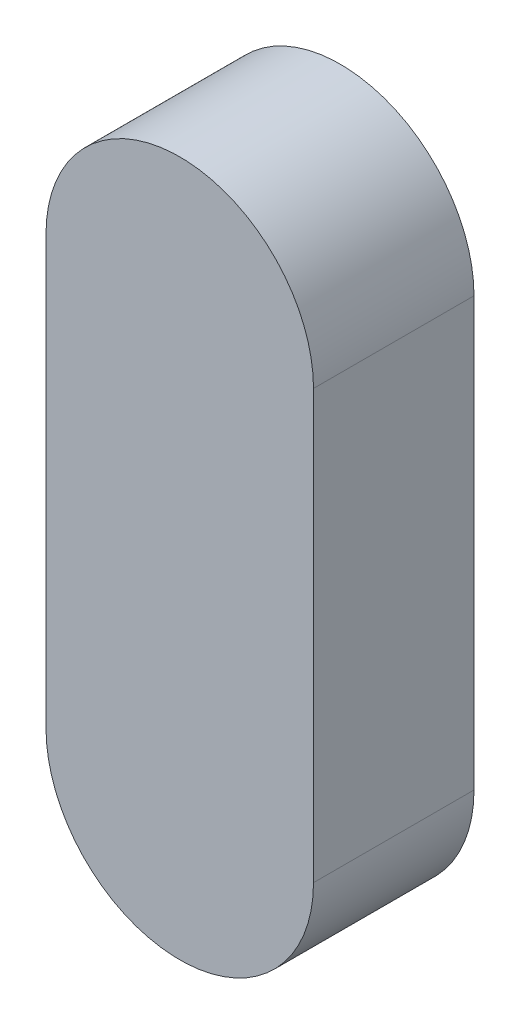
SolidWorks part; units mm, degrees
material "Plain Carbon Steel"
ref_plane "Front Plane" through (0, 0, 0) normal (0, 0, 1) x (1, 0, 0)
ref_plane "Top Plane" through (0, 0, 0) normal (0, 1, 0) x (1, 0, 0)
ref_plane "Right Plane" through (0, 0, 0) normal (1, 0, 0) x (0, 0, -1)
sketch "Key Profile 5x13" plane through (0, 0, 0) normal (0, 0, 1) x (1, 0, 0)
  line L0 (0, 28.7291) -> (0, -26.7586) construction
  line L1 (42.2463, 0) -> (-31.0542, 0) construction
  line L2 (0, 0) -> (0, 8) construction
  line L3 (-2.5, 0) -> (-2.5, 8)
  line L4 (2.5, 0) -> (2.5, 8)
  arc A0 (-2.5, 0) -> (2.5, 0) centre (0, 0) ccw
  arc A1 (2.5, 8) -> (-2.5, 8) centre (0, 8) ccw
  point P7 (0, 4)
  dimension "D2" = 2.5
  dimension "D1" = 8
extrude "Key Body 3mm" add sketch "Key Profile 5x13" along normal blind 3
